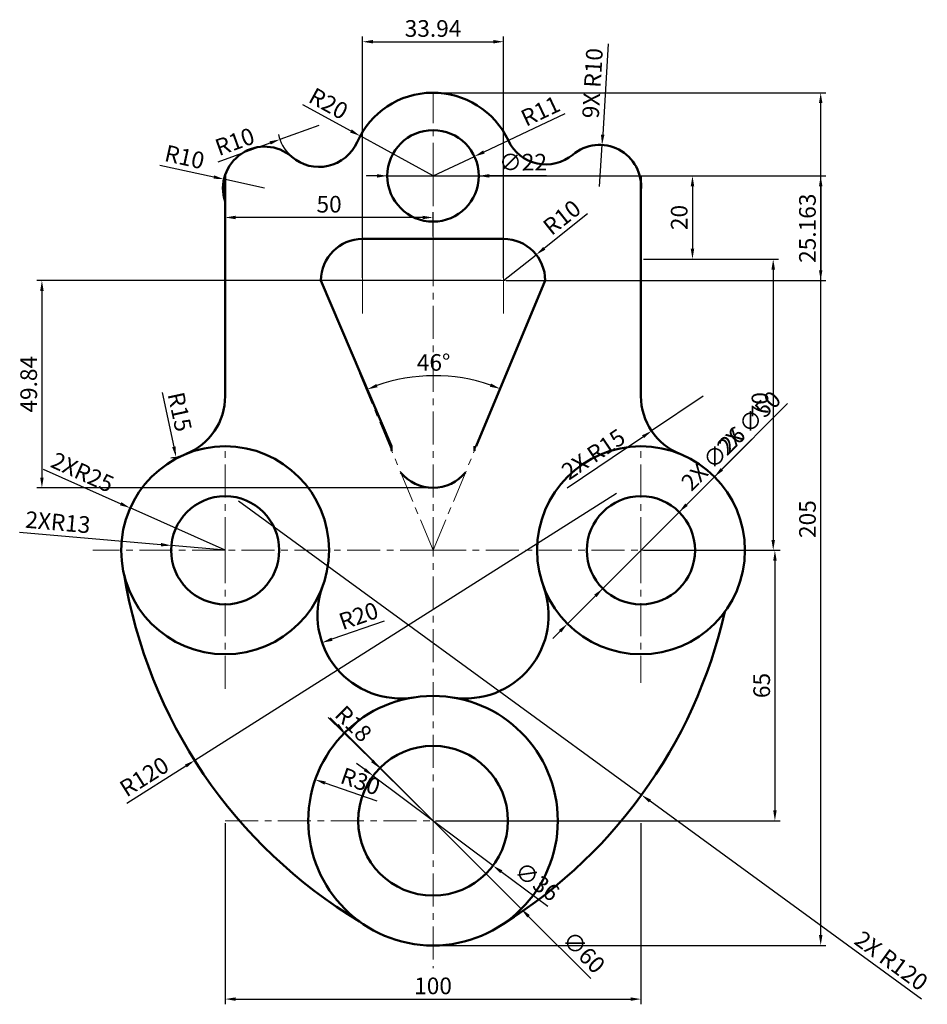
# Model space of a CAD drawing. Units: millimetres. Extents: x 2293 to 2511, y 975 to 1212.
import ezdxf

# ---------------------------------------------------------------- set-up
doc = ezdxf.new("R2010")
doc.units = ezdxf.units.MM
doc.linetypes.add('CENTER', pattern=[50.8, 31.75, -6.35, 6.35, -6.35])
for name, color, linetype, lineweight in [('M-CNTR', 4, 'CENTER', 18), ('M-CONS', 8, 'CENTER', 18), ('M-DIMS', 2, 'Continuous', 25), ('M-OUTL', 7, 'Continuous', 50)]:
    doc.layers.add(name, color=color, linetype=linetype, lineweight=lineweight)
doc.styles.get("Standard").update_dxf_attribs({"font": 'arial.ttf'})
doc.dimstyles.new('ISO-25', dxfattribs={"dimtxt": 4, "dimasz": 2.5, "dimexe": 1.25, "dimexo": 0.625, "dimtad": 1, "dimtxsty": 'Standard', "dimcen": 2.5, "dimadec": 0, "dimazin": 0, "dimtfac": 1, "dimtmove": 0, "dimatfit": 3, "dimfxl": 1, "dimarcsym": 0})

# ---------------------------------------------------------------- blocks, each defined once
blk = doc.blocks.new('*D1')
at = {"layer": 'Defpoints', "color": 0, "transparency": 16777216}
for p in [(2442.47, 1174.39), (2442.47, 1154.39), (2454.86, 1154.39)]:
    blk.add_point(p, dxfattribs=at)
at = {"layer": 'M-DIMS', "color": 0, "lineweight": -2, "transparency": 16777216}
for p, q in [((2443.1, 1174.39), (2456.11, 1174.39)), ((2454.86, 1171.89), (2454.86, 1156.89)), ((2443.1, 1154.39), (2456.11, 1154.39))]:
    blk.add_line(p, q, dxfattribs=at)
at = {"layer": 'M-DIMS', "color": 0, "transparency": 16777216}
for points in [[(2454.44, 1171.89), (2455.28, 1171.89), (2454.86, 1174.39)], [(2454.44, 1156.89), (2455.28, 1156.89), (2454.86, 1154.39)]]:
    blk.add_solid(points, dxfattribs=at)
at = {"layer": 'M-DIMS', "color": 0, "transparency": 16777216, "insert": (2452.19, 1164.39), "char_height": 4, "attachment_point": 5, "rotation": 90}
blk.add_mtext('20', dxfattribs=at)
blk = doc.blocks.new('*D2')
at = {"layer": 'Defpoints', "color": 0, "transparency": 16777216}
for p in [(2442.47, 1154.39), (2442.47, 1084.39), (2474.28, 1084.39)]:
    blk.add_point(p, dxfattribs=at)
at = {"layer": 'M-DIMS', "color": 0, "lineweight": -2, "transparency": 16777216}
for p, q in [((2443.1, 1154.39), (2475.53, 1154.39)), ((2474.28, 1151.89), (2474.28, 1086.89)), ((2443.1, 1084.39), (2475.53, 1084.39))]:
    blk.add_line(p, q, dxfattribs=at)
at = {"layer": 'M-DIMS', "color": 0, "transparency": 16777216}
for points in [[(2473.86, 1151.89), (2474.7, 1151.89), (2474.28, 1154.39)], [(2473.86, 1086.89), (2474.7, 1086.89), (2474.28, 1084.39)]]:
    blk.add_solid(points, dxfattribs=at)
at = {"layer": 'M-DIMS', "color": 0, "transparency": 16777216, "insert": (2471.61, 1119.39), "char_height": 4, "attachment_point": 5, "rotation": 90}
blk.add_mtext('70', dxfattribs=at)
blk = doc.blocks.new('*D3')
at = {"layer": 'Defpoints', "color": 0, "transparency": 16777216}
for p in [(2442.47, 1084.39), (2392.47, 1019.39), (2474.69, 1019.39)]:
    blk.add_point(p, dxfattribs=at)
at = {"layer": 'M-DIMS', "color": 0, "lineweight": -2, "transparency": 16777216}
for p, q in [((2443.1, 1084.39), (2475.94, 1084.39)), ((2474.69, 1081.89), (2474.69, 1021.89)), ((2393.1, 1019.39), (2475.94, 1019.39))]:
    blk.add_line(p, q, dxfattribs=at)
at = {"layer": 'M-DIMS', "color": 0, "transparency": 16777216}
for points in [[(2474.28, 1081.89), (2475.11, 1081.89), (2474.69, 1084.39)], [(2474.28, 1021.89), (2475.11, 1021.89), (2474.69, 1019.39)]]:
    blk.add_solid(points, dxfattribs=at)
at = {"layer": 'M-DIMS', "color": 0, "transparency": 16777216, "insert": (2472.03, 1051.89), "char_height": 4, "attachment_point": 5, "rotation": 90}
blk.add_mtext('65', dxfattribs=at)
blk = doc.blocks.new('*D4')
at = {"layer": 'Defpoints', "color": 0, "transparency": 16777216}
for p in [(2342.47, 1019.39), (2442.47, 1019.39), (2442.47, 976.52)]:
    blk.add_point(p, dxfattribs=at)
at = {"layer": 'M-DIMS', "color": 0, "lineweight": -2, "transparency": 16777216}
for p, q in [((2342.47, 1018.77), (2342.47, 975.27)), ((2442.47, 1018.77), (2442.47, 975.27)), ((2344.97, 976.52), (2439.97, 976.52))]:
    blk.add_line(p, q, dxfattribs=at)
at = {"layer": 'M-DIMS', "color": 0, "transparency": 16777216}
for points in [[(2344.97, 976.93), (2344.97, 976.1), (2342.47, 976.52)], [(2439.97, 976.93), (2439.97, 976.1), (2442.47, 976.52)]]:
    blk.add_solid(points, dxfattribs=at)
at = {"layer": 'M-DIMS', "color": 0, "transparency": 16777216, "insert": (2392.47, 979.18), "char_height": 4, "attachment_point": 5}
blk.add_mtext('100', dxfattribs=at)
blk = doc.blocks.new('*D5')
at = {"layer": 'Defpoints', "color": 0, "transparency": 16777216}
for p in [(2402.43, 1179.07), (2392.47, 1174.39)]:
    blk.add_point(p, dxfattribs=at)
at = {"layer": 'M-DIMS', "color": 0, "lineweight": -2, "transparency": 16777216}
for p, q in [((2424.17, 1189.27), (2404.69, 1180.13)), ((2392.47, 1174.39), (2402.43, 1179.07))]:
    blk.add_line(p, q, dxfattribs=at)
at = {"layer": 'M-DIMS', "color": 0, "transparency": 16777216}
blk.add_solid([(2404.52, 1180.51), (2404.87, 1179.75), (2402.43, 1179.07)], dxfattribs=at)
at = {"layer": 'M-DIMS', "color": 0, "transparency": 16777216, "insert": (2418.51, 1189.52), "char_height": 4, "attachment_point": 5, "rotation": 25.1369}
blk.add_mtext('R11', dxfattribs=at)
blk = doc.blocks.new('*D6')
at = {"layer": 'Defpoints', "color": 0, "transparency": 16777216}
for p in [(2374.93, 1183.99), (2392.47, 1174.39)]:
    blk.add_point(p, dxfattribs=at)
at = {"layer": 'M-DIMS', "color": 0, "lineweight": -2, "transparency": 16777216}
for p, q in [((2361.07, 1191.57), (2372.73, 1185.19)), ((2392.47, 1174.39), (2374.93, 1183.99))]:
    blk.add_line(p, q, dxfattribs=at)
at = {"layer": 'M-DIMS', "color": 0, "transparency": 16777216}
blk.add_solid([(2372.93, 1185.56), (2372.53, 1184.82), (2374.93, 1183.99)], dxfattribs=at)
at = {"layer": 'M-DIMS', "color": 0, "transparency": 16777216, "insert": (2367.08, 1191.32), "char_height": 4, "attachment_point": 5, "rotation": 331.3277}
blk.add_mtext('R20', dxfattribs=at)
blk = doc.blocks.new('*D7')
at = {"layer": 'Defpoints', "color": 0, "transparency": 16777216}
for p in [(2365.04, 1186.54), (2355.64, 1183.16)]:
    blk.add_point(p, dxfattribs=at)
at = {"layer": 'M-DIMS', "color": 0, "lineweight": -2, "transparency": 16777216}
for p, q in [((2365.04, 1186.54), (2355.64, 1183.16)), ((2340.78, 1177.8), (2353.28, 1182.31))]:
    blk.add_line(p, q, dxfattribs=at)
blk.add_arc((2365.04, 1186.54), 10, 192.6444, 225.5327, dxfattribs=at)
at = {"layer": 'M-DIMS', "color": 0, "transparency": 16777216}
blk.add_solid([(2353.14, 1182.7), (2353.42, 1181.92), (2355.64, 1183.16)], dxfattribs=at)
at = {"layer": 'M-DIMS', "color": 0, "transparency": 16777216, "insert": (2344.95, 1182.14), "char_height": 4, "attachment_point": 5, "rotation": 19.8064}
blk.add_mtext('R10', dxfattribs=at)
blk = doc.blocks.new('*D8')
at = {"layer": 'Defpoints', "color": 0, "transparency": 16777216}
for p in [(2342.19, 1173.59), (2351.95, 1171.42)]:
    blk.add_point(p, dxfattribs=at)
at = {"layer": 'M-DIMS', "color": 0, "lineweight": -2, "transparency": 16777216}
for p, q in [((2326.77, 1177), (2339.75, 1174.13)), ((2351.95, 1171.42), (2342.19, 1173.59))]:
    blk.add_line(p, q, dxfattribs=at)
at = {"layer": 'M-DIMS', "color": 0, "transparency": 16777216}
blk.add_solid([(2339.84, 1174.53), (2339.66, 1173.72), (2342.19, 1173.59)], dxfattribs=at)
at = {"layer": 'M-DIMS', "color": 0, "transparency": 16777216, "insert": (2332.61, 1178.44), "char_height": 4, "attachment_point": 5, "rotation": 347.516}
blk.add_mtext('R10', dxfattribs=at)
blk = doc.blocks.new('*D9')
at = {"layer": 'Defpoints', "color": 0, "transparency": 16777216}
for p in [(2417.28, 1155.45), (2409.44, 1149.23)]:
    blk.add_point(p, dxfattribs=at)
at = {"layer": 'M-DIMS', "color": 0, "lineweight": -2, "transparency": 16777216}
for p, q in [((2429.65, 1165.26), (2419.24, 1157)), ((2409.44, 1149.23), (2417.28, 1155.45))]:
    blk.add_line(p, q, dxfattribs=at)
at = {"layer": 'M-DIMS', "color": 0, "transparency": 16777216}
blk.add_solid([(2418.98, 1157.33), (2419.5, 1156.67), (2417.28, 1155.45)], dxfattribs=at)
at = {"layer": 'M-DIMS', "color": 0, "transparency": 16777216, "insert": (2423.77, 1164), "char_height": 4, "attachment_point": 5, "rotation": 38.4271}
blk.add_mtext('R10', dxfattribs=at)
blk = doc.blocks.new('*D10')
at = {"layer": 'Defpoints', "color": 0, "transparency": 16777216}
for p in [(2327.47, 1121.48), (2330.67, 1106.82)]:
    blk.add_point(p, dxfattribs=at)
at = {"layer": 'M-DIMS', "color": 0, "lineweight": -2, "transparency": 16777216}
blk.add_line((2327.29, 1122.29), (2330.14, 1109.26), dxfattribs=at)
blk.add_arc((2327.47, 1121.48), 15, 277.5292, 289.637, dxfattribs=at)
at = {"layer": 'M-DIMS', "color": 0, "transparency": 16777216}
blk.add_solid([(2330.54, 1109.35), (2329.73, 1109.17), (2330.67, 1106.82)], dxfattribs=at)
at = {"layer": 'M-DIMS', "color": 0, "transparency": 16777216, "insert": (2331.06, 1117.57), "char_height": 4, "attachment_point": 5, "rotation": 282.3038}
blk.add_mtext('R15', dxfattribs=at)
blk = doc.blocks.new('*D11')
at = {"layer": 'Defpoints', "color": 0, "transparency": 16777216}
for p in [(2319.64, 1094.57), (2342.47, 1084.39)]:
    blk.add_point(p, dxfattribs=at)
at = {"layer": 'M-DIMS', "color": 0, "lineweight": -2, "transparency": 16777216}
for p, q in [((2298.67, 1103.91), (2317.35, 1095.59)), ((2342.47, 1084.39), (2319.64, 1094.57))]:
    blk.add_line(p, q, dxfattribs=at)
at = {"layer": 'M-DIMS', "color": 0, "transparency": 16777216}
blk.add_solid([(2317.52, 1095.97), (2317.18, 1095.21), (2319.64, 1094.57)], dxfattribs=at)
at = {"layer": 'M-DIMS', "color": 0, "transparency": 16777216, "insert": (2307.96, 1102.69), "char_height": 4, "attachment_point": 5, "rotation": 335.9868}
blk.add_mtext('2XR25', dxfattribs=at)
blk = doc.blocks.new('*D12')
at = {"layer": 'Defpoints', "color": 0, "transparency": 16777216}
for p in [(2329.52, 1085.54), (2342.47, 1084.39)]:
    blk.add_point(p, dxfattribs=at)
at = {"layer": 'M-DIMS', "color": 0, "lineweight": -2, "transparency": 16777216}
for p, q in [((2293.05, 1088.76), (2327.03, 1085.76)), ((2342.47, 1084.39), (2329.52, 1085.54))]:
    blk.add_line(p, q, dxfattribs=at)
at = {"layer": 'M-DIMS', "color": 0, "transparency": 16777216}
blk.add_solid([(2327.07, 1086.17), (2327, 1085.34), (2329.52, 1085.54)], dxfattribs=at)
at = {"layer": 'M-DIMS', "color": 0, "transparency": 16777216, "insert": (2302.21, 1090.63), "char_height": 4, "attachment_point": 5, "rotation": 354.9466}
blk.add_mtext('2XR13', dxfattribs=at)
blk = doc.blocks.new('*D13')
at = {"layer": 'Defpoints', "color": 0, "transparency": 16777216}
for p in [(2436.57, 1098.03), (2335.15, 1033.9)]:
    blk.add_point(p, dxfattribs=at)
at = {"layer": 'M-DIMS', "color": 0, "lineweight": -2, "transparency": 16777216}
for p, q in [((2436.57, 1098.03), (2335.15, 1033.9)), ((2318.83, 1023.58), (2333.04, 1032.56))]:
    blk.add_line(p, q, dxfattribs=at)
at = {"layer": 'M-DIMS', "color": 0, "transparency": 16777216}
blk.add_solid([(2332.82, 1032.91), (2333.26, 1032.21), (2335.15, 1033.9)], dxfattribs=at)
at = {"layer": 'M-DIMS', "color": 0, "transparency": 16777216, "insert": (2323.28, 1029.55), "char_height": 4, "attachment_point": 5, "rotation": 32.3078}
blk.add_mtext('R120', dxfattribs=at)
blk = doc.blocks.new('*D14')
at = {"layer": 'Defpoints', "color": 0, "transparency": 16777216}
for p in [(2379.65, 1032.02), (2392.47, 1019.39)]:
    blk.add_point(p, dxfattribs=at)
at = {"layer": 'M-DIMS', "color": 0, "lineweight": -2, "transparency": 16777216}
for p, q in [((2367.24, 1044.24), (2377.87, 1033.78)), ((2392.47, 1019.39), (2379.65, 1032.02))]:
    blk.add_line(p, q, dxfattribs=at)
at = {"layer": 'M-DIMS', "color": 0, "transparency": 16777216}
blk.add_solid([(2378.16, 1034.07), (2377.57, 1033.48), (2379.65, 1032.02)], dxfattribs=at)
at = {"layer": 'M-DIMS', "color": 0, "transparency": 16777216, "insert": (2372.97, 1042.34), "char_height": 4, "attachment_point": 5, "rotation": 315.4416}
blk.add_mtext('R18', dxfattribs=at)
blk = doc.blocks.new('*D15')
at = {"layer": 'Defpoints', "color": 0, "transparency": 16777216}
for p in [(2364.15, 1029.27), (2392.47, 1019.39)]:
    blk.add_point(p, dxfattribs=at)
at = {"layer": 'M-DIMS', "color": 0, "lineweight": -2, "transparency": 16777216}
blk.add_line((2379.06, 1024.07), (2366.51, 1028.45), dxfattribs=at)
at = {"layer": 'M-DIMS', "color": 0, "transparency": 16777216}
blk.add_solid([(2366.64, 1028.84), (2366.37, 1028.06), (2364.15, 1029.27)], dxfattribs=at)
at = {"layer": 'M-DIMS', "color": 0, "transparency": 16777216, "insert": (2374.84, 1028.37), "char_height": 4, "attachment_point": 5, "rotation": 340.7776}
blk.add_mtext('R30', dxfattribs=at)
blk = doc.blocks.new('*D16')
at = {"layer": 'Defpoints', "color": 0, "transparency": 16777216}
for p in [(2342.47, 1164.39), (2342.47, 1159.23), (2392.47, 1159.23)]:
    blk.add_point(p, dxfattribs=at)
at = {"layer": 'M-DIMS', "color": 0, "lineweight": -2, "transparency": 16777216}
for p, q in [((2342.47, 1159.86), (2342.47, 1165.64)), ((2392.47, 1159.86), (2392.47, 1165.64)), ((2389.97, 1164.39), (2344.97, 1164.39))]:
    blk.add_line(p, q, dxfattribs=at)
at = {"layer": 'M-DIMS', "color": 0, "transparency": 16777216}
for points in [[(2344.97, 1164.81), (2344.97, 1163.98), (2342.47, 1164.39)], [(2389.97, 1164.81), (2389.97, 1163.98), (2392.47, 1164.39)]]:
    blk.add_solid(points, dxfattribs=at)
at = {"layer": 'M-DIMS', "color": 0, "transparency": 16777216, "insert": (2367.47, 1167.06), "char_height": 4, "attachment_point": 5}
blk.add_mtext('50', dxfattribs=at)
blk = doc.blocks.new('*D17')
at = {"layer": 'Defpoints', "color": 0, "transparency": 16777216}
for p in [(2365.5, 1149.23), (2419.44, 1149.23), (2398.08, 1126.03), (2382.47, 1109.39), (2402.87, 1109.39)]:
    blk.add_point(p, dxfattribs=at)
at = {"layer": 'M-DIMS', "color": 0, "lineweight": -2, "transparency": 16777216}
blk.add_arc((2392.79, 1085.17), 41.2, 70.8908, 109.5973, dxfattribs=at)
at = {"layer": 'M-DIMS', "color": 0, "transparency": 16777216}
for points in [[(2379.13, 1123.59), (2378.82, 1124.37), (2376.65, 1123.07)], [(2406.43, 1124.49), (2406.13, 1123.71), (2408.62, 1123.21)]]:
    blk.add_solid(points, dxfattribs=at)
at = {"layer": 'M-DIMS', "color": 0, "transparency": 16777216, "insert": (2392.61, 1129.03), "char_height": 4, "attachment_point": 5, "rotation": 0.244}
blk.add_mtext('46°', dxfattribs=at)
blk = doc.blocks.new('*D18')
at = {"layer": 'Defpoints', "color": 0, "transparency": 16777216}
for p in [(2384.68, 1068.78), (2365.79, 1062.2)]:
    blk.add_point(p, dxfattribs=at)
at = {"layer": 'M-DIMS', "color": 0, "lineweight": -2, "transparency": 16777216}
blk.add_line((2380.71, 1067.4), (2368.15, 1063.03), dxfattribs=at)
at = {"layer": 'M-DIMS', "color": 0, "transparency": 16777216}
blk.add_solid([(2368.02, 1063.42), (2368.29, 1062.63), (2365.79, 1062.2)], dxfattribs=at)
at = {"layer": 'M-DIMS', "color": 0, "transparency": 16777216, "insert": (2374.73, 1068.14), "char_height": 4, "attachment_point": 5, "rotation": 19.2032}
blk.add_mtext('R20', dxfattribs=at)
blk = doc.blocks.new('SIDE-MOUNT-OD50-BORE26')
for radius in [25, 13]:
    blk.add_circle((0, 0), radius)
blk = doc.blocks.new('*D20')
at = {"layer": 'Defpoints', "color": 0, "transparency": 16777216}
for p in [(2392.47, 1194.39), (2485.7, 1194.39), (2392.47, 989.39)]:
    blk.add_point(p, dxfattribs=at)
at = {"layer": 'M-DIMS', "color": 0, "lineweight": -2, "transparency": 16777216}
for p, q in [((2393.1, 1194.39), (2486.95, 1194.39)), ((2485.7, 991.89), (2485.7, 1191.89)), ((2393.1, 989.39), (2486.95, 989.39))]:
    blk.add_line(p, q, dxfattribs=at)
at = {"layer": 'M-DIMS', "color": 0, "transparency": 16777216}
for points in [[(2485.29, 1191.89), (2486.12, 1191.89), (2485.7, 1194.39)], [(2485.29, 991.89), (2486.12, 991.89), (2485.7, 989.39)]]:
    blk.add_solid(points, dxfattribs=at)
at = {"layer": 'M-DIMS', "color": 0, "transparency": 16777216, "insert": (2483.04, 1091.89), "char_height": 4, "attachment_point": 5, "rotation": 90}
blk.add_mtext('205', dxfattribs=at)
blk = doc.blocks.new('*D21')
at = {"layer": 'Defpoints', "color": 0, "transparency": 16777216}
for p in [(2409.44, 1206.64), (2375.5, 1149.23), (2409.44, 1149.23)]:
    blk.add_point(p, dxfattribs=at)
at = {"layer": 'M-DIMS', "color": 0, "lineweight": -2, "transparency": 16777216}
for p, q in [((2375.5, 1149.86), (2375.5, 1207.89)), ((2409.44, 1149.86), (2409.44, 1207.89)), ((2378, 1206.64), (2406.94, 1206.64))]:
    blk.add_line(p, q, dxfattribs=at)
at = {"layer": 'M-DIMS', "color": 0, "transparency": 16777216}
for points in [[(2378, 1207.06), (2378, 1206.23), (2375.5, 1206.64)], [(2406.94, 1207.06), (2406.94, 1206.23), (2409.44, 1206.64)]]:
    blk.add_solid(points, dxfattribs=at)
at = {"layer": 'M-DIMS', "color": 0, "transparency": 16777216, "insert": (2392.47, 1209.31), "char_height": 4, "attachment_point": 5}
blk.add_mtext('33.94', dxfattribs=at)
blk = doc.blocks.new('*D22')
at = {"layer": 'Defpoints', "color": 0, "transparency": 16777216}
for p in [(2392.47, 1174.39), (2409.44, 1149.23), (2485.7, 1149.23)]:
    blk.add_point(p, dxfattribs=at)
at = {"layer": 'M-DIMS', "color": 0, "lineweight": -2, "transparency": 16777216}
for p, q in [((2393.1, 1174.39), (2486.95, 1174.39)), ((2485.7, 1171.89), (2485.7, 1151.73)), ((2410.07, 1149.23), (2486.95, 1149.23))]:
    blk.add_line(p, q, dxfattribs=at)
at = {"layer": 'M-DIMS', "color": 0, "transparency": 16777216}
for points in [[(2485.29, 1171.89), (2486.12, 1171.89), (2485.7, 1174.39)], [(2485.29, 1151.73), (2486.12, 1151.73), (2485.7, 1149.23)]]:
    blk.add_solid(points, dxfattribs=at)
at = {"layer": 'M-DIMS', "color": 0, "transparency": 16777216, "insert": (2483.03, 1161.81), "char_height": 4, "attachment_point": 5, "rotation": 90}
blk.add_mtext('25.163', dxfattribs=at)
blk = doc.blocks.new('*D23')
at = {"layer": 'Defpoints', "color": 0, "transparency": 16777216}
for p in [(2409.44, 1149.23), (2298.4, 1099.39), (2392.47, 1099.39)]:
    blk.add_point(p, dxfattribs=at)
at = {"layer": 'M-DIMS', "color": 0, "lineweight": -2, "transparency": 16777216}
for p, q in [((2408.82, 1149.23), (2297.15, 1149.23)), ((2298.4, 1146.73), (2298.4, 1101.89)), ((2391.85, 1099.39), (2297.15, 1099.39))]:
    blk.add_line(p, q, dxfattribs=at)
at = {"layer": 'M-DIMS', "color": 0, "transparency": 16777216}
for points in [[(2297.99, 1146.73), (2298.82, 1146.73), (2298.4, 1149.23)], [(2297.99, 1101.89), (2298.82, 1101.89), (2298.4, 1099.39)]]:
    blk.add_solid(points, dxfattribs=at)
at = {"layer": 'M-DIMS', "color": 0, "transparency": 16777216, "insert": (2295.74, 1124.31), "char_height": 4, "attachment_point": 5, "rotation": 90}
blk.add_mtext('49.84', dxfattribs=at)
blk = doc.blocks.new('*D24')
at = {"layer": 'Defpoints', "color": 0, "transparency": 16777216}
for p in [(2371.26, 1040.61), (2413.69, 998.18)]:
    blk.add_point(p, dxfattribs=at)
at = {"layer": 'M-DIMS', "color": 0, "lineweight": -2, "transparency": 16777216}
for p, q in [((2369.49, 1042.38), (2367.72, 1044.14)), ((2371.26, 1040.61), (2413.69, 998.18)), ((2430.42, 981.45), (2415.45, 996.41))]:
    blk.add_line(p, q, dxfattribs=at)
at = {"layer": 'M-DIMS', "color": 0, "transparency": 16777216}
for points in [[(2369.79, 1042.67), (2369.2, 1042.08), (2371.26, 1040.61)], [(2415.75, 996.71), (2415.16, 996.12), (2413.69, 998.18)]]:
    blk.add_solid(points, dxfattribs=at)
at = {"layer": 'M-DIMS', "color": 0, "transparency": 16777216, "insert": (2428.38, 987.42), "char_height": 4, "attachment_point": 5, "rotation": 315.0005}
blk.add_mtext('∅60', dxfattribs=at)
blk = doc.blocks.new('*D25')
at = {"layer": 'Defpoints', "color": 0, "transparency": 16777216}
for p in [(2378.06, 1030.18), (2406.89, 1008.61)]:
    blk.add_point(p, dxfattribs=at)
at = {"layer": 'M-DIMS', "color": 0, "lineweight": -2, "transparency": 16777216}
for p, q in [((2376.06, 1031.68), (2374.06, 1033.17)), ((2378.06, 1030.18), (2406.89, 1008.61)), ((2420.07, 998.75), (2408.89, 1007.11))]:
    blk.add_line(p, q, dxfattribs=at)
at = {"layer": 'M-DIMS', "color": 0, "transparency": 16777216}
for points in [[(2376.31, 1032.01), (2375.81, 1031.34), (2378.06, 1030.18)], [(2409.14, 1007.45), (2408.64, 1006.78), (2406.89, 1008.61)]]:
    blk.add_solid(points, dxfattribs=at)
at = {"layer": 'M-DIMS', "color": 0, "transparency": 16777216, "insert": (2417.2, 1004.37), "char_height": 4, "attachment_point": 5, "rotation": 323.1953}
blk.add_mtext('∅36', dxfattribs=at)
blk = doc.blocks.new('*D26')
at = {"layer": 'Defpoints', "color": 0, "transparency": 16777216}
for p in [(2460.15, 1102.07), (2424.79, 1066.72)]:
    blk.add_point(p, dxfattribs=at)
at = {"layer": 'M-DIMS', "color": 0, "lineweight": -2, "transparency": 16777216}
for p, q in [((2477.75, 1119.67), (2461.92, 1103.84)), ((2424.79, 1066.72), (2460.15, 1102.07)), ((2423.03, 1064.95), (2421.26, 1063.18))]:
    blk.add_line(p, q, dxfattribs=at)
at = {"layer": 'M-DIMS', "color": 0, "transparency": 16777216}
for points in [[(2461.62, 1104.13), (2462.21, 1103.54), (2460.15, 1102.07)], [(2422.73, 1065.24), (2423.32, 1064.66), (2424.79, 1066.72)]]:
    blk.add_solid(points, dxfattribs=at)
at = {"layer": 'M-DIMS', "color": 0, "transparency": 16777216, "insert": (2468.79, 1114.64), "char_height": 4, "attachment_point": 5, "rotation": 44.9976}
blk.add_mtext('2X ∅50', dxfattribs=at)
blk = doc.blocks.new('*D27')
at = {"layer": 'Defpoints', "color": 0, "transparency": 16777216}
for p in [(2451.66, 1093.59), (2433.28, 1075.2)]:
    blk.add_point(p, dxfattribs=at)
at = {"layer": 'M-DIMS', "color": 0, "lineweight": -2, "transparency": 16777216}
for p, q in [((2469.17, 1111.12), (2453.43, 1095.36)), ((2433.28, 1075.2), (2451.66, 1093.59)), ((2431.52, 1073.43), (2429.75, 1071.66))]:
    blk.add_line(p, q, dxfattribs=at)
at = {"layer": 'M-DIMS', "color": 0, "transparency": 16777216}
for points in [[(2453.13, 1095.65), (2453.72, 1095.07), (2451.66, 1093.59)], [(2431.22, 1073.72), (2431.81, 1073.13), (2433.28, 1075.2)]]:
    blk.add_solid(points, dxfattribs=at)
at = {"layer": 'M-DIMS', "color": 0, "transparency": 16777216, "insert": (2460.22, 1106.09), "char_height": 4, "attachment_point": 5, "rotation": 45.0265}
blk.add_mtext('2X ∅26', dxfattribs=at)
blk = doc.blocks.new('*D28')
at = {"layer": 'Defpoints', "color": 0, "transparency": 16777216}
for p in [(2381.47, 1174.39), (2403.47, 1174.39)]:
    blk.add_point(p, dxfattribs=at)
at = {"layer": 'M-DIMS', "color": 0, "lineweight": -2, "transparency": 16777216}
for p, q in [((2378.97, 1174.39), (2376.47, 1174.39)), ((2381.47, 1174.39), (2403.47, 1174.39)), ((2419.76, 1174.4), (2405.97, 1174.39))]:
    blk.add_line(p, q, dxfattribs=at)
at = {"layer": 'M-DIMS', "color": 0, "transparency": 16777216}
for points in [[(2378.97, 1174.81), (2378.97, 1173.98), (2381.47, 1174.39)], [(2405.97, 1174.81), (2405.97, 1173.98), (2403.47, 1174.39)]]:
    blk.add_solid(points, dxfattribs=at)
at = {"layer": 'M-DIMS', "color": 0, "transparency": 16777216, "insert": (2414.12, 1177.17), "char_height": 4, "attachment_point": 5, "rotation": 0.0022}
blk.add_mtext('∅22', dxfattribs=at)
blk = doc.blocks.new('*D29')
at = {"layer": 'Defpoints', "color": 0, "transparency": 16777216}
for p in [(2345.67, 1096.3), (2442.63, 1025.6)]:
    blk.add_point(p, dxfattribs=at)
at = {"layer": 'M-DIMS', "color": 0, "lineweight": -2, "transparency": 16777216}
for p, q in [((2345.67, 1096.3), (2442.63, 1025.6)), ((2509.92, 976.53), (2444.65, 1024.12))]:
    blk.add_line(p, q, dxfattribs=at)
at = {"layer": 'M-DIMS', "color": 0, "transparency": 16777216}
blk.add_solid([(2444.89, 1024.46), (2444.4, 1023.79), (2442.63, 1025.6)], dxfattribs=at)
at = {"layer": 'M-DIMS', "color": 0, "transparency": 16777216, "insert": (2502.38, 985.33), "char_height": 4, "attachment_point": 5, "rotation": 323.9025}
blk.add_mtext('2X R120', dxfattribs=at)
blk = doc.blocks.new('*D30')
at = {"layer": 'Defpoints', "color": 0, "transparency": 16777216}
for p in [(2457.47, 1121.48), (2445.04, 1113.09)]:
    blk.add_point(p, dxfattribs=at)
at = {"layer": 'M-DIMS', "color": 0, "lineweight": -2, "transparency": 16777216}
for p, q in [((2457.47, 1121.48), (2445.04, 1113.09)), ((2424.72, 1099.39), (2442.96, 1111.69))]:
    blk.add_line(p, q, dxfattribs=at)
at = {"layer": 'M-DIMS', "color": 0, "transparency": 16777216}
blk.add_solid([(2442.73, 1112.04), (2443.2, 1111.35), (2445.04, 1113.09)], dxfattribs=at)
at = {"layer": 'M-DIMS', "color": 0, "transparency": 16777216, "insert": (2431.31, 1107.06), "char_height": 4, "attachment_point": 5, "rotation": 33.9894}
blk.add_mtext('2X R15', dxfattribs=at)
blk = doc.blocks.new('*D31')
at = {"layer": 'Defpoints', "color": 0, "transparency": 16777216}
for p in [(2433.12, 1181.82), (2432.52, 1171.84)]:
    blk.add_point(p, dxfattribs=at)
at = {"layer": 'M-DIMS', "color": 0, "lineweight": -2, "transparency": 16777216}
for p, q in [((2434.59, 1206.17), (2433.27, 1184.32)), ((2432.52, 1171.84), (2433.12, 1181.82))]:
    blk.add_line(p, q, dxfattribs=at)
at = {"layer": 'M-DIMS', "color": 0, "transparency": 16777216}
blk.add_solid([(2432.85, 1184.34), (2433.69, 1184.29), (2433.12, 1181.82)], dxfattribs=at)
at = {"layer": 'M-DIMS', "color": 0, "transparency": 16777216, "insert": (2431.34, 1196.65), "char_height": 4, "attachment_point": 5, "rotation": 86.5416}
blk.add_mtext('9X R10', dxfattribs=at)

msp = doc.modelspace()

# ---------------------------------------------------------------- linework, layer by layer
at = {"layer": 'M-CNTR', "ltscale": 0.25}
for p, q in [((2392.4731, 1174.3946), (2392.4731, 1194.3946)), ((2376.3517, 1174.3946), (2409.4076, 1174.3946)), ((2392.4731, 1154.3946), (2392.4731, 1174.3946)), ((2375.5023, 1149.2313), (2375.5023, 1159.2313)), ((2409.4439, 1149.2313), (2409.4439, 1159.2313)), ((2392.4731, 1084.3946), (2392.4731, 1154.3946)), ((2360.6502, 1149.2313), (2425.9355, 1149.2313)), ((2375.5023, 1149.2313), (2375.5023, 1141.2726)), ((2409.4439, 1149.2313), (2409.4439, 1140.8597)), ((2342.4731, 1084.3946), (2342.4731, 1109.3946)), ((2442.4731, 1084.3946), (2442.4731, 1109.3946)), ((2342.4731, 1084.3946), (2310.6532, 1084.3946)), ((2392.4731, 1084.3946), (2342.4731, 1084.3946)), ((2342.4731, 1084.3946), (2342.4731, 1050.454)), ((2392.4731, 1019.3946), (2392.4731, 1084.3946)), ((2392.4731, 1084.3946), (2442.4731, 1084.3946)), ((2442.4731, 1084.3946), (2473.4533, 1084.3946)), ((2442.4731, 1084.3946), (2442.4731, 1052.518)), ((2342.4731, 1019.3946), (2442.4731, 1019.3946)), ((2392.4731, 1019.3946), (2392.4731, 983.9913))]:
    msp.add_line(p, q, dxfattribs=at)
at = {"layer": 'M-CONS', "ltscale": 0.25}
for q in [(2365.5023, 1149.2313), (2419.4439, 1149.2313)]:
    msp.add_line((2392.4731, 1084.3946), q, dxfattribs=at)
at = {"layer": 'M-OUTL'}
for p, q in [((2342.4731, 1154.3946), (2342.4731, 1174.3946)), ((2442.4731, 1154.3946), (2442.4731, 1174.3946)), ((2375.5023, 1159.2313), (2409.4439, 1159.2313)), ((2342.4731, 1121.4756), (2342.4731, 1154.3946)), ((2442.4731, 1121.4756), (2442.4731, 1154.3946)), ((2382.4731, 1109.3946), (2365.5023, 1149.2313)), ((2402.8726, 1109.3946), (2419.4439, 1149.2313))]:
    msp.add_line(p, q, dxfattribs=at)
for centre, radius in [((2392.4731, 1174.3946), 11), ((2392.4731, 1019.3946), 30), ((2392.4731, 1019.3946), 18)]:
    msp.add_circle(centre, radius, dxfattribs=at)
for centre, radius, start, end in [((2392.4731, 1174.3946), 20, 25.136869, 156.108446), ((2351.9525, 1171.4246), 10, 49.113675, 198.569475), ((2365.0437, 1186.5448), 10, 229.113675, 336.108446), ((2419.6319, 1187.138), 10, 205.136869, 310.107004), ((2432.5163, 1171.8412), 10, 354.671612, 130.107004), ((2375.5023, 1149.2313), 10, 90, 180), ((2409.4439, 1149.2313), 10, 0, 90), ((2327.4731, 1121.4756), 15, 292.024313, 0), ((2457.4731, 1121.4756), 15, 180, 247.975687), ((2392.4731, 1109.3946), 10, 180, 186.364643), ((2392.4731, 1109.3946), 10, 353.635357, 0), ((2392.4731, 1109.3946), 10, 218.808035, 321.191965), ((2436.5739, 1098.0338), 120, 189.346212, 239.006618), ((2384.6784, 1068.7833), 20, 159.701077, 278.968654), ((2400.2678, 1068.7833), 20, 261.031346, 20.298923), ((2345.6658, 1096.2966), 120, 300.627202, 347.177851)]:
    msp.add_arc(centre, radius, start, end, dxfattribs=at)

# ---------------------------------------------------------------- block references
for p in [(2342.4731, 1084.3946), (2442.4731, 1084.3946)]:
    msp.add_blockref('SIDE-MOUNT-OD50-BORE26', p, dxfattribs=at)

# ---------------------------------------------------------------- dimensions: what is measured, and where the dimension line sits
at = {"layer": 'M-DIMS'}
for base, p1, p2, override, picture, middle in [((2409.4439, 1206.6446), (2375.5023, 1149.2313), (2409.4439, 1149.2313), {"dimdec": 2, "dimlfac": 1, "dimrnd": 0, "dimzin": 0, "dimdsep": 46, "dimlunit": 2}, '*D21', (2392.4731, 1209.3132)), ((2342.4731, 1164.3946), (2392.4731, 1159.2313), (2342.4731, 1159.2313), {"dimclrd": 0, "dimclre": 0, "dimclrt": 0}, '*D16', (2367.4731, 1167.0619)), ((2442.4731, 976.5162), (2342.4731, 1019.3946), (2442.4731, 1019.3946), {"dimclrd": 0, "dimclre": 0, "dimclrt": 0}, '*D4', (2392.4731, 979.1835))]:
    dim = msp.add_linear_dim(base=base, p1=p1, p2=p2, dimstyle='ISO-25', override=override, dxfattribs=at)
    dim.commit()
    dim.dimension.update_dxf_attribs({"geometry": picture, "text_midpoint": middle})
for center, mpoint, text, override, picture, middle in [((2432.5163, 1171.8412), (2433.1195, 1181.823), '9X <>', {"dimdec": 0, "dimlfac": 1, "dimrnd": 0, "dimzin": 0, "dimdsep": 46, "dimlunit": 2}, '*D31', (2431.3435, 1196.6517)), ((2457.4731, 1121.4756), (2445.036, 1113.09), '2X <>', {"dimdec": 0, "dimlfac": 1, "dimrnd": 0, "dimzin": 0, "dimdsep": 46, "dimlunit": 2}, '*D30', (2431.3146, 1107.0554)), ((2342.4731, 1084.3946), (2319.6368, 1094.5683), '2X<>', {"dimclrd": 0, "dimclre": 0, "dimclrt": 0}, '*D11', (2307.9574, 1102.6915))]:
    dim = msp.add_radius_dim(center=center, mpoint=mpoint, text=text, dimstyle='ISO-25', override=override, dxfattribs=at)
    dim.commit()
    dim.dimension.update_dxf_attribs({"geometry": picture, "text_midpoint": middle})
for center, mpoint, picture, middle in [((2392.4731, 1174.3946), (2374.9255, 1183.9906), '*D6', (2367.083, 1191.3194)), ((2365.0437, 1186.5448), (2355.6352, 1183.1563), '*D7', (2344.9493, 1182.1428)), ((2351.9525, 1171.4246), (2342.1889, 1173.5863), '*D8', (2332.6141, 1178.438)), ((2409.4439, 1149.2313), (2417.2779, 1155.4465), '*D9', (2423.7652, 1163.9981))]:
    dim = msp.add_radius_dim(center=center, mpoint=mpoint, dimstyle='ISO-25', override={"dimclrd": 0, "dimclre": 0, "dimclrt": 0}, dxfattribs=at)
    dim.commit()
    dim.dimension.update_dxf_attribs({"geometry": picture, "text_midpoint": middle})
for base, p1, p2, override, picture, middle in [((2485.7033, 1194.3946), (2392.4731, 989.3946), (2392.4731, 1194.3946), {"dimdec": 0, "dimlfac": 1, "dimrnd": 0, "dimzin": 0, "dimdsep": 46, "dimlunit": 2}, '*D20', (2483.036, 1091.8946)), ((2485.7033, 1149.2313), (2392.4731, 1174.3946), (2409.4439, 1149.2313), {"dimdec": 3, "dimlfac": 1, "dimrnd": 0, "dimzin": 0, "dimdsep": 46, "dimlunit": 2}, '*D22', (2483.0346, 1161.8129)), ((2454.8594, 1154.3946), (2442.4731, 1174.3946), (2442.4731, 1154.3946), {"dimclrd": 0, "dimclre": 0, "dimclrt": 0}, '*D1', (2452.1921, 1164.3946)), ((2474.2797, 1084.3946), (2442.4731, 1154.3946), (2442.4731, 1084.3946), {"dimclrd": 0, "dimclre": 0, "dimclrt": 0}, '*D2', (2471.6124, 1119.3946)), ((2298.4032, 1099.3946), (2409.4439, 1149.2313), (2392.4731, 1099.3946), {"dimdec": 2, "dimlfac": 1, "dimrnd": 0, "dimzin": 0, "dimdsep": 46, "dimlunit": 2}, '*D23', (2295.7359, 1124.3129)), ((2474.6929, 1019.3946), (2442.4731, 1084.3946), (2392.4731, 1019.3946), {"dimclrd": 0, "dimclre": 0, "dimclrt": 0}, '*D3', (2472.0256, 1051.8946))]:
    dim = msp.add_linear_dim(base=base, p1=p1, p2=p2, angle=90, dimstyle='ISO-25', override=override, dxfattribs=at)
    dim.commit()
    dim.dimension.update_dxf_attribs({"geometry": picture, "text_midpoint": middle})
for center, mpoint, picture, middle in [((2392.4731, 1174.3946), (2402.4313, 1179.0672), '*D5', (2419.6319, 1187.138)), ((2327.4731, 1121.4756), (2330.6695, 1106.8201), '*D10', (2328.4493, 1116.9998)), ((2436.5739, 1098.0338), (2335.1512, 1033.8977), '*D13', (2324.7053, 1027.292)), ((2384.6784, 1068.7833), (2365.7912, 1062.2049), '*D18', (2375.6099, 1065.6247)), ((2392.4731, 1019.3946), (2379.6474, 1032.024), '*D14', (2371.097, 1040.4436)), ((2392.4731, 1019.3946), (2364.1456, 1029.2716), '*D15', (2373.9631, 1025.8485))]:
    dim = msp.add_radius_dim(center=center, mpoint=mpoint, dimstyle='ISO-25', override={"dimclrd": 0, "dimclre": 0, "dimclrt": 0}, dxfattribs=at)
    dim.commit()
    dim.dimension.update_dxf_attribs({"geometry": picture, "text_midpoint": middle, "dimtype": 164})
dim = msp.add_diameter_dim_2p(p1=(2381.4731, 1174.3941), p2=(2403.4731, 1174.395), dimstyle='ISO-25', override={"dimdec": 0, "dimlfac": 1, "dimrnd": 0, "dimzin": 0, "dimdsep": 46, "dimlunit": 2}, dxfattribs=at)
dim.commit()
dim.dimension.update_dxf_attribs({"geometry": '*D28', "text_midpoint": (2414.1185, 1174.3954)})
dim = msp.add_angular_dim_2l(base=(2398.0767, 1126.0281), line1=((2402.8726, 1109.3946), (2419.4439, 1149.2313)), line2=((2382.4731, 1109.3946), (2365.5023, 1149.2313)), dimstyle='ISO-25', override={"dimclrd": 0, "dimclre": 0, "dimclrt": 0}, dxfattribs=at)
dim.commit()
dim.dimension.update_dxf_attribs({"geometry": '*D17', "text_midpoint": (2392.6075, 1129.035)})
dim = msp.add_diameter_dim_2p(p1=(2424.7947, 1066.7177), p2=(2460.1515, 1102.0715), text='2X <>', dimstyle='ISO-25', override={"dimdec": 0, "dimlfac": 1, "dimrnd": 0, "dimzin": 0, "dimdsep": 46, "dimlunit": 2}, dxfattribs=at)
dim.commit()
dim.dimension.update_dxf_attribs({"geometry": '*D26', "text_midpoint": (2470.7585, 1112.6776), "dimtype": 163})
dim = msp.add_diameter_dim_2p(p1=(2433.2849, 1075.1979), p2=(2451.6612, 1093.5912), text='2X <>', dimstyle='ISO-25', override={"dimdec": 0, "dimlfac": 1, "dimrnd": 0, "dimzin": 0, "dimdsep": 46, "dimlunit": 2}, dxfattribs=at)
dim.commit()
dim.dimension.update_dxf_attribs({"geometry": '*D27', "text_midpoint": (2462.1849, 1104.1247)})
for center, mpoint, text, override, picture, middle in [((2345.6658, 1096.2966), (2442.6277, 1025.5972), '2X <>', {"dimdec": 0, "dimlfac": 1, "dimrnd": 0, "dimzin": 0, "dimdsep": 46, "dimlunit": 2}, '*D29', (2500.8048, 983.1776)), ((2342.4731, 1084.3946), (2329.5236, 1085.5397), '2X<>', {"dimclrd": 0, "dimclre": 0, "dimclrt": 0}, '*D12', (2301.9794, 1087.9753))]:
    dim = msp.add_radius_dim(center=center, mpoint=mpoint, text=text, dimstyle='ISO-25', override=override, dxfattribs=at)
    dim.commit()
    dim.dimension.update_dxf_attribs({"geometry": picture, "text_midpoint": middle, "dimtype": 164})
for p1, p2, picture, middle in [((2371.2597, 1040.6076), (2413.6865, 998.1815), '*D24', (2426.4145, 985.4537)), ((2378.0608, 1030.1782), (2406.8854, 1008.611), '*D25', (2415.5327, 1002.1408))]:
    dim = msp.add_diameter_dim_2p(p1=p1, p2=p2, dimstyle='ISO-25', override={"dimdec": 0, "dimlfac": 1, "dimrnd": 0, "dimzin": 0, "dimdsep": 46, "dimlunit": 2}, dxfattribs=at)
    dim.commit()
    dim.dimension.update_dxf_attribs({"geometry": picture, "text_midpoint": middle, "dimtype": 163})

doc.saveas('drawing.dxf')
